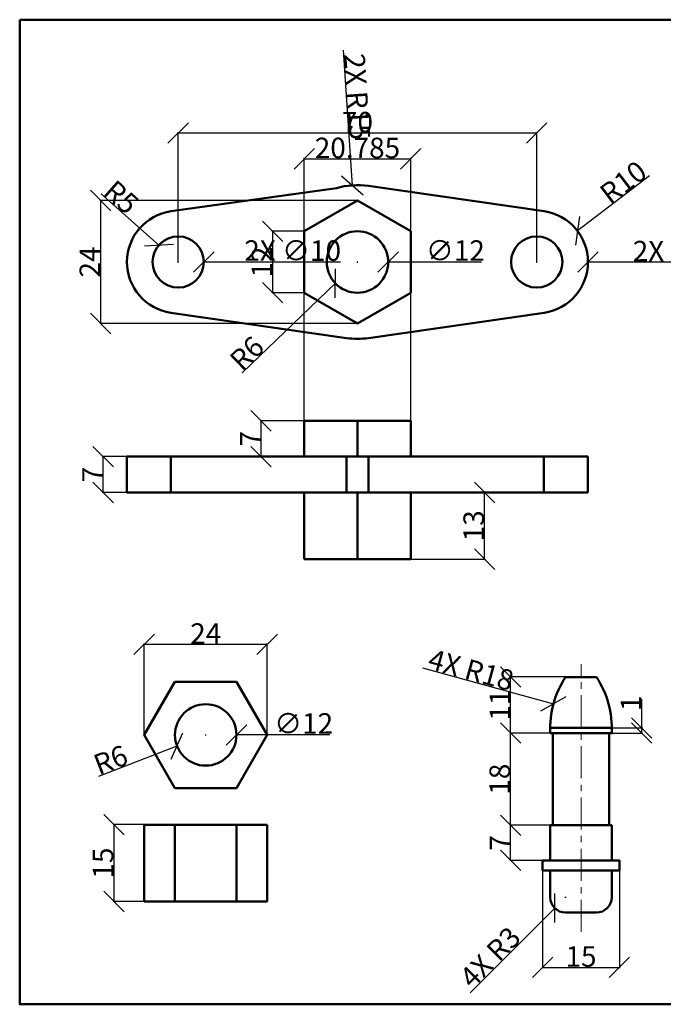
# Model space of a CAD drawing. Units: millimetres. Extents: x 4 to 224, y 3 to 195.
# Tile 1 of 2: x 4 to 129, y 3 to 195. Entities that reach past the tile are written whole.
import ezdxf

# ---------------------------------------------------------------- set-up
doc = ezdxf.new("R2010")
doc.units = ezdxf.units.MM
doc.header["$MEASUREMENT"] = 0
doc.linetypes.add('CENTER', pattern=[2, 1.25, -0.25, 0.25, -0.25])
for name, color, linetype, lineweight in [('M-CNTR', 1, 'CENTER', 18), ('M-DIMS', 2, 'Continuous', 25), ('M-OUTL', 7, 'Continuous', 50)]:
    doc.layers.add(name, color=color, linetype=linetype, lineweight=lineweight)
doc.styles.get("Standard").update_dxf_attribs({"font": 'arial.ttf'})
doc.dimstyles.get("Standard").update_dxf_attribs({"dimtxt": 4, "dimasz": 4, "dimexe": 0.18, "dimexo": 0.0625, "dimgap": 0.09, "dimtad": 1, "dimdec": 0, "dimzin": 0, "dimdsep": 46, "dimtxsty": 'Standard', "dimblk": 'OBLIQUE', "dimcen": 0.09, "dimclre": 251, "dimadec": 0, "dimazin": 0, "dimtfac": 1, "dimtdec": 0, "dimtofl": 0, "dimtmove": 0, "dimatfit": 3, "dimfxl": 1, "dimtolj": 1, "dimtzin": 0, "dimarcsym": 0})

# ---------------------------------------------------------------- blocks, each defined once
blk = doc.blocks.new('_Oblique')
at = {"color": 0, "linetype": 'ByBlock', "lineweight": -2}
blk.add_line((-0.5, -0.5), (0.5, 0.5), dxfattribs=at)
blk = doc.blocks.new('*D2')
at = {"layer": 'Defpoints', "color": 0, "transparency": 16777216}
for p in [(104.72, 173.13), (34.72, 147.94), (104.72, 147.94)]:
    blk.add_point(p, dxfattribs=at)
at = {"layer": 'M-DIMS', "color": 0, "lineweight": -2, "transparency": 16777216}
for p, q in [((34.72, 148.01), (34.72, 173.31)), ((34.72, 173.13), (104.72, 173.13)), ((104.72, 148.01), (104.72, 173.31))]:
    blk.add_line(p, q, dxfattribs=at)
at = {"layer": 'M-DIMS', "color": 0, "lineweight": -2, "transparency": 16777216, "xscale": 4, "yscale": 4, "zscale": 4, "rotation": 180}
blk.add_blockref('_Oblique', (34.72, 173.13), dxfattribs=at)
at = {"layer": 'M-DIMS', "color": 0, "lineweight": -2, "transparency": 16777216, "xscale": 4, "yscale": 4, "zscale": 4}
blk.add_blockref('_Oblique', (104.72, 173.13), dxfattribs=at)
at = {"layer": 'M-DIMS', "color": 0, "transparency": 16777216, "insert": (69.72, 175.26), "char_height": 4, "attachment_point": 5}
blk.add_mtext('\\A1;70', dxfattribs=at)
blk = doc.blocks.new('*D3')
at = {"layer": 'Defpoints', "color": 0, "transparency": 16777216}
for p in [(59.33, 153.94), (53.16, 141.94), (59.33, 141.94)]:
    blk.add_point(p, dxfattribs=at)
at = {"layer": 'M-DIMS', "color": 0, "lineweight": -2, "transparency": 16777216}
for p, q in [((59.27, 153.94), (52.98, 153.94)), ((53.16, 153.94), (53.16, 141.94)), ((59.27, 141.94), (52.98, 141.94))]:
    blk.add_line(p, q, dxfattribs=at)
at = {"layer": 'M-DIMS', "color": 0, "lineweight": -2, "transparency": 16777216, "xscale": 4, "yscale": 4, "zscale": 4}
for p, rotation in [((53.16, 153.94), 90), ((53.16, 141.94), 270)]:
    blk.add_blockref('_Oblique', p, dxfattribs=dict(at, rotation=rotation))
at = {"layer": 'M-DIMS', "color": 0, "transparency": 16777216, "insert": (51.06, 147.94), "char_height": 4, "attachment_point": 5, "rotation": 90}
blk.add_mtext('\\A1;12', dxfattribs=at)
blk = doc.blocks.new('*D4')
at = {"layer": 'Defpoints', "color": 0, "transparency": 16777216}
for p in [(69.72, 147.94), (65.4, 143.78)]:
    blk.add_point(p, dxfattribs=at)
at = {"layer": 'M-DIMS', "color": 0, "lineweight": -2, "transparency": 16777216}
for p, q in [((69.72, 147.85), (69.72, 148.03)), ((69.63, 147.94), (69.81, 147.94)), ((47.22, 126.29), (65.4, 143.78))]:
    blk.add_line(p, q, dxfattribs=at)
at = {"layer": 'M-DIMS', "color": 0, "lineweight": -2, "transparency": 16777216, "xscale": 4, "yscale": 4, "zscale": 4, "rotation": 43.89831917731966}
blk.add_blockref('_Oblique', (65.4, 143.78), dxfattribs=at)
at = {"layer": 'M-DIMS', "color": 0, "transparency": 16777216, "insert": (48.13, 130.13), "char_height": 4, "attachment_point": 5, "rotation": 43.8983}
blk.add_mtext('\\A1;R6', dxfattribs=at)
blk = doc.blocks.new('*D5')
at = {"layer": 'Defpoints', "color": 0, "transparency": 16777216}
for p in [(112.67, 154.01), (104.72, 147.94)]:
    blk.add_point(p, dxfattribs=at)
at = {"layer": 'M-DIMS', "color": 0, "lineweight": -2, "transparency": 16777216}
for p, q in [((126.76, 164.76), (112.67, 154.01)), ((104.72, 147.85), (104.72, 148.03)), ((104.63, 147.94), (104.81, 147.94))]:
    blk.add_line(p, q, dxfattribs=at)
at = {"layer": 'M-DIMS', "color": 0, "lineweight": -2, "transparency": 16777216, "xscale": 4, "yscale": 4, "zscale": 4, "rotation": 217.3494381917111}
blk.add_blockref('_Oblique', (112.67, 154.01), dxfattribs=at)
at = {"layer": 'M-DIMS', "color": 0, "transparency": 16777216, "insert": (121.6, 163.51), "char_height": 4, "attachment_point": 5, "rotation": 37.3494}
blk.add_mtext('\\A1;R10', dxfattribs=at)
blk = doc.blocks.new('*D6')
at = {"layer": 'Defpoints', "color": 0, "transparency": 16777216}
for p in [(30.97, 151.26), (34.72, 147.94)]:
    blk.add_point(p, dxfattribs=at)
at = {"layer": 'M-DIMS', "color": 0, "lineweight": -2, "transparency": 16777216}
for p, q in [((19.69, 161.23), (30.97, 151.26)), ((34.72, 147.85), (34.72, 148.03)), ((34.63, 147.94), (34.81, 147.94))]:
    blk.add_line(p, q, dxfattribs=at)
at = {"layer": 'M-DIMS', "color": 0, "lineweight": -2, "transparency": 16777216, "xscale": 4, "yscale": 4, "zscale": 4, "rotation": 318.5221166633732}
blk.add_blockref('_Oblique', (30.97, 151.26), dxfattribs=at)
at = {"layer": 'M-DIMS', "color": 0, "transparency": 16777216, "insert": (23.6, 160.61), "char_height": 4, "attachment_point": 5, "rotation": 318.5221}
blk.add_mtext('\\A1;R5', dxfattribs=at)
blk = doc.blocks.new('*D7')
at = {"layer": 'Defpoints', "color": 0, "transparency": 16777216}
for p in [(20.08, 109.94), (24.72, 109.94), (24.72, 102.94)]:
    blk.add_point(p, dxfattribs=at)
at = {"layer": 'M-DIMS', "color": 0, "lineweight": -2, "transparency": 16777216}
for p, q in [((24.66, 109.94), (19.9, 109.94)), ((20.08, 102.94), (20.08, 109.94)), ((24.66, 102.94), (19.9, 102.94))]:
    blk.add_line(p, q, dxfattribs=at)
at = {"layer": 'M-DIMS', "color": 0, "lineweight": -2, "transparency": 16777216, "xscale": 4, "yscale": 4, "zscale": 4}
for p, rotation in [((20.08, 109.94), 90), ((20.08, 102.94), 270)]:
    blk.add_blockref('_Oblique', p, dxfattribs=dict(at, rotation=rotation))
at = {"layer": 'M-DIMS', "color": 0, "transparency": 16777216, "insert": (17.99, 106.44), "char_height": 4, "attachment_point": 5, "rotation": 90}
blk.add_mtext('\\A1;7', dxfattribs=at)
blk = doc.blocks.new('*D8')
at = {"layer": 'Defpoints', "color": 0, "transparency": 16777216}
for p in [(59.33, 116.94), (50.88, 109.94), (50.88, 109.94)]:
    blk.add_point(p, dxfattribs=at)
at = {"layer": 'M-DIMS', "color": 0, "lineweight": -2, "transparency": 16777216}
for p, q in [((59.27, 116.94), (50.7, 116.94)), ((50.88, 116.94), (50.88, 109.94)), ((50.81, 109.94), (50.7, 109.94))]:
    blk.add_line(p, q, dxfattribs=at)
at = {"layer": 'M-DIMS', "color": 0, "lineweight": -2, "transparency": 16777216, "xscale": 4, "yscale": 4, "zscale": 4}
for p, rotation in [((50.88, 116.94), 90), ((50.88, 109.94), 270)]:
    blk.add_blockref('_Oblique', p, dxfattribs=dict(at, rotation=rotation))
at = {"layer": 'M-DIMS', "color": 0, "transparency": 16777216, "insert": (48.79, 113.44), "char_height": 4, "attachment_point": 5, "rotation": 90}
blk.add_mtext('\\A1;7', dxfattribs=at)
blk = doc.blocks.new('*D9')
at = {"layer": 'Defpoints', "color": 0, "transparency": 16777216}
for p in [(94.54, 102.94), (94.54, 102.94), (80.11, 89.94)]:
    blk.add_point(p, dxfattribs=at)
at = {"layer": 'M-DIMS', "color": 0, "lineweight": -2, "transparency": 16777216}
for p, q in [((94.54, 89.94), (94.54, 102.94)), ((94.6, 102.94), (94.72, 102.94)), ((80.17, 89.94), (94.72, 89.94))]:
    blk.add_line(p, q, dxfattribs=at)
at = {"layer": 'M-DIMS', "color": 0, "lineweight": -2, "transparency": 16777216, "xscale": 4, "yscale": 4, "zscale": 4}
for p, rotation in [((94.54, 102.94), 90), ((94.54, 89.94), 270)]:
    blk.add_blockref('_Oblique', p, dxfattribs=dict(at, rotation=rotation))
at = {"layer": 'M-DIMS', "color": 0, "transparency": 16777216, "insert": (92.41, 96.44), "char_height": 4, "attachment_point": 5, "rotation": 90}
blk.add_mtext('\\A1;13', dxfattribs=at)
blk = doc.blocks.new('*D22')
at = {"layer": 'Defpoints', "color": 0, "transparency": 16777216}
for p in [(52.09, 73.3), (28.09, 55.61), (52.09, 55.61)]:
    blk.add_point(p, dxfattribs=at)
at = {"layer": 'M-DIMS', "color": 0, "lineweight": -2, "transparency": 16777216}
for p, q in [((28.09, 55.67), (28.09, 73.48)), ((28.09, 73.3), (52.09, 73.3)), ((52.09, 55.67), (52.09, 73.48))]:
    blk.add_line(p, q, dxfattribs=at)
at = {"layer": 'M-DIMS', "color": 0, "lineweight": -2, "transparency": 16777216, "xscale": 4, "yscale": 4, "zscale": 4, "rotation": 180}
blk.add_blockref('_Oblique', (28.09, 73.3), dxfattribs=at)
at = {"layer": 'M-DIMS', "color": 0, "lineweight": -2, "transparency": 16777216, "xscale": 4, "yscale": 4, "zscale": 4}
blk.add_blockref('_Oblique', (52.09, 73.3), dxfattribs=at)
at = {"layer": 'M-DIMS', "color": 0, "transparency": 16777216, "insert": (40.09, 75.4), "char_height": 4, "attachment_point": 5}
blk.add_mtext('\\A1;24', dxfattribs=at)
blk = doc.blocks.new('*D23')
at = {"layer": 'Defpoints', "color": 0, "transparency": 16777216}
for p in [(40.09, 55.61), (34.5, 53.45)]:
    blk.add_point(p, dxfattribs=at)
at = {"layer": 'M-DIMS', "color": 0, "lineweight": -2, "transparency": 16777216}
for p, q in [((40, 55.61), (40.18, 55.61)), ((40.09, 55.52), (40.09, 55.7)), ((19.21, 47.57), (34.5, 53.45))]:
    blk.add_line(p, q, dxfattribs=at)
at = {"layer": 'M-DIMS', "color": 0, "lineweight": -2, "transparency": 16777216, "xscale": 4, "yscale": 4, "zscale": 4, "rotation": 21.05754839460186}
blk.add_blockref('_Oblique', (34.5, 53.45), dxfattribs=at)
at = {"layer": 'M-DIMS', "color": 0, "transparency": 16777216, "insert": (21.53, 50.75), "char_height": 4, "attachment_point": 5, "rotation": 21.0575}
blk.add_mtext('\\A1;R6', dxfattribs=at)
blk = doc.blocks.new('*D24')
at = {"layer": 'Defpoints', "color": 0, "transparency": 16777216}
for p in [(28.09, 38.09), (22.18, 23.09), (28.09, 23.09)]:
    blk.add_point(p, dxfattribs=at)
at = {"layer": 'M-DIMS', "color": 0, "lineweight": -2, "transparency": 16777216}
for p, q in [((28.03, 38.09), (22, 38.09)), ((22.18, 38.09), (22.18, 23.09)), ((28.03, 23.09), (22, 23.09))]:
    blk.add_line(p, q, dxfattribs=at)
at = {"layer": 'M-DIMS', "color": 0, "lineweight": -2, "transparency": 16777216, "xscale": 4, "yscale": 4, "zscale": 4}
for p, rotation in [((22.18, 38.09), 90), ((22.18, 23.09), 270)]:
    blk.add_blockref('_Oblique', p, dxfattribs=dict(at, rotation=rotation))
at = {"layer": 'M-DIMS', "color": 0, "transparency": 16777216, "insert": (20.05, 30.59), "char_height": 4, "attachment_point": 5, "rotation": 90}
blk.add_mtext('\\A1;15', dxfattribs=at)
blk = doc.blocks.new('*D25')
at = {"layer": 'Defpoints', "color": 0, "transparency": 16777216}
for p in [(105.86, 29.12), (120.86, 29.12), (120.86, 10.22)]:
    blk.add_point(p, dxfattribs=at)
at = {"layer": 'M-DIMS', "color": 0, "lineweight": -2, "transparency": 16777216}
for p, q in [((105.86, 29.05), (105.86, 10.04)), ((120.86, 29.05), (120.86, 10.04)), ((105.86, 10.22), (120.86, 10.22))]:
    blk.add_line(p, q, dxfattribs=at)
at = {"layer": 'M-DIMS', "color": 0, "lineweight": -2, "transparency": 16777216, "xscale": 4, "yscale": 4, "zscale": 4, "rotation": 180}
blk.add_blockref('_Oblique', (105.86, 10.22), dxfattribs=at)
at = {"layer": 'M-DIMS', "color": 0, "lineweight": -2, "transparency": 16777216, "xscale": 4, "yscale": 4, "zscale": 4}
blk.add_blockref('_Oblique', (120.86, 10.22), dxfattribs=at)
at = {"layer": 'M-DIMS', "color": 0, "transparency": 16777216, "insert": (113.36, 12.35), "char_height": 4, "attachment_point": 5}
blk.add_mtext('\\A1;15', dxfattribs=at)
blk = doc.blocks.new('*D26')
at = {"layer": 'Defpoints', "color": 0, "transparency": 16777216}
for p in [(99.62, 37.97), (107.36, 37.97), (105.86, 31.12)]:
    blk.add_point(p, dxfattribs=at)
at = {"layer": 'M-DIMS', "color": 0, "lineweight": -2, "transparency": 16777216}
for p, q in [((107.3, 37.97), (99.44, 37.97)), ((99.62, 31.12), (99.62, 37.97)), ((105.8, 31.12), (99.44, 31.12))]:
    blk.add_line(p, q, dxfattribs=at)
at = {"layer": 'M-DIMS', "color": 0, "lineweight": -2, "transparency": 16777216, "xscale": 4, "yscale": 4, "zscale": 4}
for p, rotation in [((99.62, 37.97), 90), ((99.62, 31.12), 270)]:
    blk.add_blockref('_Oblique', p, dxfattribs=dict(at, rotation=rotation))
at = {"layer": 'M-DIMS', "color": 0, "transparency": 16777216, "insert": (97.53, 34.54), "char_height": 4, "attachment_point": 5, "rotation": 90}
blk.add_mtext('\\A1;7', dxfattribs=at)
blk = doc.blocks.new('*D27')
at = {"layer": 'Defpoints', "color": 0, "transparency": 16777216}
for p in [(99.62, 55.97), (107.36, 55.97), (107.36, 37.97)]:
    blk.add_point(p, dxfattribs=at)
at = {"layer": 'M-DIMS', "color": 0, "lineweight": -2, "transparency": 16777216}
for p, q in [((107.3, 55.97), (99.44, 55.97)), ((99.62, 37.97), (99.62, 55.97)), ((107.3, 37.97), (99.44, 37.97))]:
    blk.add_line(p, q, dxfattribs=at)
at = {"layer": 'M-DIMS', "color": 0, "lineweight": -2, "transparency": 16777216, "xscale": 4, "yscale": 4, "zscale": 4}
for p, rotation in [((99.62, 55.97), 90), ((99.62, 37.97), 270)]:
    blk.add_blockref('_Oblique', p, dxfattribs=dict(at, rotation=rotation))
at = {"layer": 'M-DIMS', "color": 0, "transparency": 16777216, "insert": (97.49, 46.97), "char_height": 4, "attachment_point": 5, "rotation": 90}
blk.add_mtext('\\A1;18', dxfattribs=at)
blk = doc.blocks.new('*D28')
at = {"layer": 'Defpoints', "color": 0, "transparency": 16777216}
for p in [(99.62, 66.92), (110.36, 66.92), (107.36, 55.97)]:
    blk.add_point(p, dxfattribs=at)
at = {"layer": 'M-DIMS', "color": 0, "lineweight": -2, "transparency": 16777216}
for p, q in [((110.3, 66.92), (99.44, 66.92)), ((99.62, 55.97), (99.62, 66.92)), ((107.3, 55.97), (99.44, 55.97))]:
    blk.add_line(p, q, dxfattribs=at)
at = {"layer": 'M-DIMS', "color": 0, "lineweight": -2, "transparency": 16777216, "xscale": 4, "yscale": 4, "zscale": 4}
for p, rotation in [((99.62, 66.92), 90), ((99.62, 55.97), 270)]:
    blk.add_blockref('_Oblique', p, dxfattribs=dict(at, rotation=rotation))
at = {"layer": 'M-DIMS', "color": 0, "transparency": 16777216, "insert": (97.52, 61.44), "char_height": 4, "attachment_point": 5, "rotation": 90}
blk.add_mtext('\\A1;11', dxfattribs=at)
blk = doc.blocks.new('*D29')
at = {"layer": 'Defpoints', "color": 0, "transparency": 16777216}
for p in [(119.36, 56.97), (119.36, 55.97), (125.22, 56.97)]:
    blk.add_point(p, dxfattribs=at)
at = {"layer": 'M-DIMS', "color": 0, "lineweight": -2, "transparency": 16777216}
for p, q in [((125.22, 56.97), (125.22, 62.62)), ((119.42, 56.97), (125.4, 56.97)), ((119.42, 55.97), (125.4, 55.97)), ((125.22, 55.97), (125.22, 56.97))]:
    blk.add_line(p, q, dxfattribs=at)
at = {"layer": 'M-DIMS', "color": 0, "lineweight": -2, "transparency": 16777216, "xscale": 4, "yscale": 4, "zscale": 4}
for p, rotation in [((125.22, 56.97), 90), ((125.22, 55.97), 270)]:
    blk.add_blockref('_Oblique', p, dxfattribs=dict(at, rotation=rotation))
at = {"layer": 'M-DIMS', "color": 0, "transparency": 16777216, "insert": (123.13, 61.79), "char_height": 4, "attachment_point": 5, "rotation": 90}
blk.add_mtext('\\A1;1', dxfattribs=at)
blk = doc.blocks.new('*D37')
at = {"layer": 'Defpoints', "color": 0, "transparency": 16777216}
for p in [(69.72, 159.94), (19.57, 135.94), (69.72, 135.94)]:
    blk.add_point(p, dxfattribs=at)
at = {"layer": 'M-DIMS', "color": 251, "lineweight": -2, "transparency": 16777216}
for p, q in [((69.66, 159.94), (19.39, 159.94)), ((69.66, 135.94), (19.39, 135.94))]:
    blk.add_line(p, q, dxfattribs=at)
at = {"layer": 'M-DIMS', "color": 0, "lineweight": -2, "transparency": 16777216}
blk.add_line((19.57, 159.94), (19.57, 135.94), dxfattribs=at)
at = {"layer": 'M-DIMS', "color": 0, "lineweight": -2, "transparency": 16777216, "xscale": 4, "yscale": 4, "zscale": 4}
for p, rotation in [((19.57, 159.94), 90), ((19.57, 135.94), 270)]:
    blk.add_blockref('_Oblique', p, dxfattribs=dict(at, rotation=rotation))
at = {"layer": 'M-DIMS', "color": 0, "transparency": 16777216, "insert": (17.47, 147.94), "char_height": 4, "attachment_point": 5, "rotation": 90}
blk.add_mtext('\\A1;24', dxfattribs=at)
blk = doc.blocks.new('*D38')
at = {"layer": 'Defpoints', "color": 0, "transparency": 16777216}
for p in [(80.11, 168.08), (59.33, 116.94), (80.11, 116.94)]:
    blk.add_point(p, dxfattribs=at)
at = {"layer": 'M-DIMS', "color": 251, "lineweight": -2, "transparency": 16777216}
for p, q in [((59.33, 117), (59.33, 168.26)), ((80.11, 117), (80.11, 168.26))]:
    blk.add_line(p, q, dxfattribs=at)
at = {"layer": 'M-DIMS', "color": 0, "lineweight": -2, "transparency": 16777216}
blk.add_line((59.33, 168.08), (80.11, 168.08), dxfattribs=at)
at = {"layer": 'M-DIMS', "color": 0, "lineweight": -2, "transparency": 16777216, "xscale": 4, "yscale": 4, "zscale": 4, "rotation": 180}
blk.add_blockref('_Oblique', (59.33, 168.08), dxfattribs=at)
at = {"layer": 'M-DIMS', "color": 0, "lineweight": -2, "transparency": 16777216, "xscale": 4, "yscale": 4, "zscale": 4}
blk.add_blockref('_Oblique', (80.11, 168.08), dxfattribs=at)
at = {"layer": 'M-DIMS', "color": 0, "transparency": 16777216, "insert": (69.72, 170.22), "char_height": 4, "attachment_point": 5}
blk.add_mtext('\\A1;20.785', dxfattribs=at)
blk = doc.blocks.new('*D40')
at = {"layer": 'Defpoints', "color": 0, "transparency": 16777216}
for p in [(29.72, 147.95), (39.72, 147.94)]:
    blk.add_point(p, dxfattribs=at)
at = {"layer": 'M-DIMS', "color": 251, "lineweight": -2, "transparency": 16777216}
for p, q in [((34.72, 147.85), (34.72, 148.03)), ((34.63, 147.94), (34.81, 147.94))]:
    blk.add_line(p, q, dxfattribs=at)
at = {"layer": 'M-DIMS', "color": 0, "lineweight": -2, "transparency": 16777216}
blk.add_line((66.42, 147.92), (39.72, 147.94), dxfattribs=at)
at = {"layer": 'M-DIMS', "color": 0, "lineweight": -2, "transparency": 16777216, "xscale": 4, "yscale": 4, "zscale": 4, "rotation": 179.9524330357494}
blk.add_blockref('_Oblique', (39.72, 147.94), dxfattribs=at)
at = {"layer": 'M-DIMS', "color": 0, "transparency": 16777216, "insert": (57.07, 150.17), "char_height": 4, "attachment_point": 5, "rotation": 359.9524}
blk.add_mtext('\\A1;2X ∅10', dxfattribs=at)
blk = doc.blocks.new('*D41')
at = {"layer": 'Defpoints', "color": 0, "transparency": 16777216}
for p in [(63.72, 147.95), (75.72, 147.94)]:
    blk.add_point(p, dxfattribs=at)
at = {"layer": 'M-DIMS', "color": 251, "lineweight": -2, "transparency": 16777216}
for p, q in [((69.72, 147.85), (69.72, 148.03)), ((69.63, 147.94), (69.81, 147.94))]:
    blk.add_line(p, q, dxfattribs=at)
at = {"layer": 'M-DIMS', "color": 0, "lineweight": -2, "transparency": 16777216}
blk.add_line((93.94, 147.93), (75.72, 147.94), dxfattribs=at)
at = {"layer": 'M-DIMS', "color": 0, "lineweight": -2, "transparency": 16777216, "xscale": 4, "yscale": 4, "zscale": 4, "rotation": 179.9603608629846}
blk.add_blockref('_Oblique', (75.72, 147.94), dxfattribs=at)
at = {"layer": 'M-DIMS', "color": 0, "transparency": 16777216, "insert": (88.83, 150.18), "char_height": 4, "attachment_point": 5, "rotation": 359.9604}
blk.add_mtext('\\A1;∅12', dxfattribs=at)
blk = doc.blocks.new('*D42')
at = {"layer": 'Defpoints', "color": 0, "transparency": 16777216}
for p in [(104.72, 147.94), (114.72, 147.94)]:
    blk.add_point(p, dxfattribs=at)
at = {"layer": 'M-DIMS', "color": 251, "lineweight": -2, "transparency": 16777216}
for p, q in [((104.72, 147.85), (104.72, 148.03)), ((104.63, 147.94), (104.81, 147.94))]:
    blk.add_line(p, q, dxfattribs=at)
at = {"layer": 'M-DIMS', "color": 0, "lineweight": -2, "transparency": 16777216}
blk.add_line((141.11, 147.93), (114.72, 147.94), dxfattribs=at)
at = {"layer": 'M-DIMS', "color": 0, "lineweight": -2, "transparency": 16777216, "xscale": 4, "yscale": 4, "zscale": 4, "rotation": 179.9762165209119}
blk.add_blockref('_Oblique', (114.72, 147.94), dxfattribs=at)
at = {"layer": 'M-DIMS', "color": 0, "transparency": 16777216, "insert": (131.91, 150.07), "char_height": 4, "attachment_point": 5, "rotation": 359.9762}
blk.add_mtext('\\A1;2X R10', dxfattribs=at)
blk = doc.blocks.new('*D43')
at = {"layer": 'Defpoints', "color": 0, "transparency": 16777216}
for p in [(68.71, 162.91), (69.72, 147.94)]:
    blk.add_point(p, dxfattribs=at)
at = {"layer": 'M-DIMS', "color": 0, "lineweight": -2, "transparency": 16777216}
blk.add_line((66.93, 189.28), (68.71, 162.91), dxfattribs=at)
at = {"layer": 'M-DIMS', "color": 251, "lineweight": -2, "transparency": 16777216}
for p, q in [((69.72, 147.85), (69.72, 148.03)), ((69.63, 147.94), (69.81, 147.94))]:
    blk.add_line(p, q, dxfattribs=at)
at = {"layer": 'M-DIMS', "color": 0, "lineweight": -2, "transparency": 16777216, "xscale": 4, "yscale": 4, "zscale": 4, "rotation": 273.8605650789521}
blk.add_blockref('_Oblique', (68.71, 162.91), dxfattribs=at)
at = {"layer": 'M-DIMS', "color": 0, "transparency": 16777216, "insert": (69.68, 180.23), "char_height": 4, "attachment_point": 5, "rotation": 273.8606}
blk.add_mtext('\\A1;2X R15', dxfattribs=at)
blk = doc.blocks.new('*D45')
at = {"layer": 'Defpoints', "color": 0, "transparency": 16777216}
for p in [(34.09, 55.61), (46.09, 55.61)]:
    blk.add_point(p, dxfattribs=at)
at = {"layer": 'M-DIMS', "color": 251, "lineweight": -2, "transparency": 16777216}
for p, q in [((40, 55.61), (40.18, 55.61)), ((40.09, 55.52), (40.09, 55.7))]:
    blk.add_line(p, q, dxfattribs=at)
at = {"layer": 'M-DIMS', "color": 0, "lineweight": -2, "transparency": 16777216}
blk.add_line((64.32, 55.61), (46.09, 55.61), dxfattribs=at)
at = {"layer": 'M-DIMS', "color": 0, "lineweight": -2, "transparency": 16777216, "xscale": 4, "yscale": 4, "zscale": 4, "rotation": 179.9944136615151}
blk.add_blockref('_Oblique', (46.09, 55.61), dxfattribs=at)
at = {"layer": 'M-DIMS', "color": 0, "transparency": 16777216, "insert": (59.21, 57.85), "char_height": 4, "attachment_point": 5, "rotation": 359.9944}
blk.add_mtext('\\A1;∅12', dxfattribs=at)
blk = doc.blocks.new('*D46')
at = {"layer": 'Defpoints', "color": 0, "transparency": 16777216}
for p in [(107.98, 61.69), (125.33, 56.93)]:
    blk.add_point(p, dxfattribs=at)
at = {"layer": 'M-DIMS', "color": 0, "lineweight": -2, "transparency": 16777216}
blk.add_line((82.42, 68.7), (107.98, 61.69), dxfattribs=at)
at = {"layer": 'M-DIMS', "color": 251, "lineweight": -2, "transparency": 16777216}
for p, q in [((125.24, 56.93), (125.42, 56.93)), ((125.33, 56.84), (125.33, 57.02))]:
    blk.add_line(p, q, dxfattribs=at)
at = {"layer": 'M-DIMS', "color": 0, "lineweight": -2, "transparency": 16777216, "xscale": 4, "yscale": 4, "zscale": 4, "rotation": 344.6657255947465}
blk.add_blockref('_Oblique', (107.98, 61.69), dxfattribs=at)
at = {"layer": 'M-DIMS', "color": 0, "transparency": 16777216, "insert": (91.9, 68.31), "char_height": 4, "attachment_point": 5, "rotation": 344.6657}
blk.add_mtext('\\A1;4X R18', dxfattribs=at)
blk = doc.blocks.new('*D47')
at = {"layer": 'Defpoints', "color": 0, "transparency": 16777216}
for p in [(110.36, 23.92), (108.24, 21.8)]:
    blk.add_point(p, dxfattribs=at)
at = {"layer": 'M-DIMS', "color": 251, "lineweight": -2, "transparency": 16777216}
for p, q in [((110.27, 23.92), (110.45, 23.92)), ((110.36, 23.83), (110.36, 24.01))]:
    blk.add_line(p, q, dxfattribs=at)
at = {"layer": 'M-DIMS', "color": 0, "lineweight": -2, "transparency": 16777216}
blk.add_line((91.69, 5.27), (108.24, 21.8), dxfattribs=at)
at = {"layer": 'M-DIMS', "color": 0, "lineweight": -2, "transparency": 16777216, "xscale": 4, "yscale": 4, "zscale": 4, "rotation": 44.95188258666079}
blk.add_blockref('_Oblique', (108.24, 21.8), dxfattribs=at)
at = {"layer": 'M-DIMS', "color": 0, "transparency": 16777216, "insert": (95.62, 12.22), "char_height": 4, "attachment_point": 5, "rotation": 44.9519}
blk.add_mtext('\\A1;4X R3', dxfattribs=at)

msp = doc.modelspace()

# ---------------------------------------------------------------- linework, layer by layer
at = {"layer": 'M-CNTR', "ltscale": 5}
msp.add_line((113.3604, 17.1404), (113.3604, 69.4089), dxfattribs=at)
at = {"layer": 'M-OUTL'}
for p, q in [((33.3328, 157.8475), (65.5987, 162.3669)), ((71.8628, 162.7903), (106.1485, 157.8416)), ((33.2913, 138.0467), (67.5771, 133.098)), ((71.8628, 133.098), (106.1485, 138.0467)), ((59.3276, 116.9392), (59.3276, 109.9392)), ((59.3276, 116.9392), (80.1122, 116.9392)), ((69.7199, 116.9392), (69.7199, 109.9392)), ((80.1122, 116.9392), (80.1122, 109.9392)), ((24.7199, 102.9392), (24.7199, 109.9392)), ((24.7199, 109.9392), (114.7199, 109.9392)), ((33.3115, 102.9392), (33.3115, 109.9392)), ((67.5558, 102.9392), (67.5558, 109.9392)), ((71.8415, 102.9392), (71.8415, 109.9392)), ((106.1272, 102.9392), (106.1272, 109.9392)), ((114.7199, 102.9392), (114.7199, 109.9392)), ((24.7199, 102.9392), (114.7199, 102.9392)), ((59.3276, 102.9392), (59.3276, 89.9392)), ((69.7199, 102.9392), (69.7199, 89.9392)), ((80.1122, 102.9392), (80.1122, 89.9392)), ((59.3276, 89.9392), (80.1122, 89.9392)), ((110.3604, 66.9169), (116.3604, 66.9169)), ((107.3604, 56.9669), (119.3604, 56.9669)), ((107.3604, 55.9669), (119.3604, 55.9669)), ((107.8604, 37.9669), (107.8604, 55.9669)), ((118.8604, 37.9669), (118.8604, 55.9669)), ((28.0945, 38.0878), (28.0945, 23.0878)), ((28.0945, 38.0878), (52.0945, 38.0878)), ((34.0945, 38.0878), (34.0945, 23.0878)), ((46.0945, 38.0878), (46.0945, 23.0878)), ((52.0945, 38.0878), (52.0945, 23.0878)), ((107.3604, 31.1169), (107.3604, 37.9669)), ((107.3604, 37.9669), (119.3604, 37.9669)), ((119.3604, 31.1169), (119.3604, 37.9669)), ((107.3604, 23.9169), (107.3604, 29.1169)), ((119.3604, 23.9169), (119.3604, 29.1169)), ((28.0945, 23.0878), (52.0945, 23.0878)), ((110.3604, 20.9169), (116.3604, 20.9169))]:
    msp.add_line(p, q, dxfattribs=at)
for points in [[(3.7754, 195.2521), (224.2583, 195.2521), (224.2583, 3.0162), (3.7754, 3.0162)], [(59.3276, 141.9442), (69.7199, 135.9442), (80.1122, 141.9442), (80.1122, 153.9442), (69.7199, 159.9442), (59.3276, 153.9442)], [(34.0945, 66.0029), (28.0945, 55.6106), (34.0945, 45.2183), (46.0945, 45.2183), (52.0945, 55.6106), (46.0945, 66.0029)], [(105.8604, 31.1169), (120.8604, 31.1169), (120.8604, 29.1169), (105.8604, 29.1169)]]:
    msp.add_lwpolyline(points, close=True, dxfattribs=at)
for centre, radius in [((69.7199, 147.9442), 6), ((34.7199, 147.9442), 5), ((104.7199, 147.9442), 5), ((40.0945, 55.6106), 6)]:
    msp.add_circle(centre, radius, dxfattribs=at)
for centre, radius, start, end in [((69.7199, 147.9442), 15, 81.786789, 105.946867), ((34.7199, 147.9442), 10, 97.973434, 261.786789), ((104.7199, 147.9442), 10, 278.213211, 81.786789), ((69.7199, 147.9442), 15, 261.786789, 278.213211), ((125.3347, 56.9284), 18, 146.294997, 183.061983), ((101.3861, 56.9284), 18, 356.938017, 33.705003), ((110.3604, 23.9169), 3, 180, 270), ((116.3604, 23.9169), 3, 270, 0)]:
    msp.add_arc(centre, radius, start, end, dxfattribs=at)

# ---------------------------------------------------------------- dimensions: what is measured, and where the dimension line sits
at = {"layer": 'M-DIMS'}
for center, mpoint, text, picture, middle in [((69.7199, 147.9442), (68.71, 162.9101), '2X <>', '*D43', (69.6783, 180.2301)), ((104.7199, 147.9442), (114.7199, 147.94), '2X <>', '*D42', (131.9145, 150.0652)), ((125.3347, 56.9284), (107.9756, 61.6885), '4X <>', '*D46', (91.9026, 68.3069)), ((110.3604, 23.9169), (108.2373, 21.7973), '4X <>', '*D47', (95.6239, 12.22))]:
    dim = msp.add_radius_dim(center=center, mpoint=mpoint, text=text, dimstyle='Standard', override={"dimdec": 0, "dimlfac": 1, "dimrnd": 0, "dimzin": 0, "dimdsep": 46, "dimlunit": 2}, dxfattribs=at)
    dim.commit()
    dim.dimension.update_dxf_attribs({"geometry": picture, "text_midpoint": middle})
for base, p1, p2, override, picture, middle in [((104.7199, 173.1324), (34.7199, 147.9442), (104.7199, 147.9442), {"dimclrd": 0, "dimclre": 0, "dimclrt": 0}, '*D2', (69.7199, 175.2647)), ((80.1122, 168.0834), (59.3276, 116.9392), (80.1122, 116.9392), {"dimdec": 3, "dimlfac": 1, "dimrnd": 0, "dimzin": 0, "dimdsep": 46, "dimlunit": 2}, '*D38', (69.7199, 170.2157)), ((52.0945, 73.301), (28.0945, 55.6106), (52.0945, 55.6106), {"dimclrd": 0, "dimclre": 0, "dimclrt": 0}, '*D22', (40.0945, 75.3992)), ((120.8604, 10.2166), (105.8604, 29.1169), (120.8604, 29.1169), {"dimclrd": 0, "dimclre": 0, "dimclrt": 0}, '*D25', (113.3604, 12.3489))]:
    dim = msp.add_linear_dim(base=base, p1=p1, p2=p2, dimstyle='Standard', override=override, dxfattribs=at)
    dim.commit()
    dim.dimension.update_dxf_attribs({"geometry": picture, "text_midpoint": middle})
dim = msp.add_radius_dim(center=(104.7199, 147.9442), mpoint=(112.6694, 154.0109), dimstyle='Standard', override={"dimclrd": 0, "dimclre": 0, "dimclrt": 0}, dxfattribs=at)
dim.commit()
dim.dimension.update_dxf_attribs({"geometry": '*D5', "text_midpoint": (121.6006, 163.5091)})
for center, mpoint, picture, middle in [((34.7199, 147.9442), (30.9739, 151.2558), '*D6', (22.1882, 159.0227)), ((69.7199, 147.9442), (65.3965, 143.7839), '*D4', (49.6091, 128.5922)), ((40.0945, 55.6106), (34.4952, 53.4548), '*D23', (22.3002, 48.7595))]:
    dim = msp.add_radius_dim(center=center, mpoint=mpoint, dimstyle='Standard', override={"dimclrd": 0, "dimclre": 0, "dimclrt": 0}, dxfattribs=at)
    dim.commit()
    dim.dimension.update_dxf_attribs({"geometry": picture, "text_midpoint": middle, "dimtype": 164})
for base, p1, p2, override, picture, middle in [((19.5699, 135.9442), (69.7199, 159.9442), (69.7199, 135.9442), {"dimdec": 0, "dimlfac": 1, "dimrnd": 0, "dimzin": 0, "dimdsep": 46, "dimlunit": 2}, '*D37', (17.4718, 147.9442)), ((53.163, 141.9442), (59.3276, 153.9442), (59.3276, 141.9442), {"dimclrd": 0, "dimclre": 0, "dimclrt": 0}, '*D3', (51.0648, 147.9442)), ((50.8755, 109.9392), (59.3276, 116.9392), (50.8755, 109.9392), {"dimclrd": 0, "dimclre": 0, "dimclrt": 0}, '*D8', (48.7855, 113.4392)), ((20.0839, 109.9392), (24.7199, 102.9392), (24.7199, 109.9392), {"dimclrd": 0, "dimclre": 0, "dimclrt": 0}, '*D7', (17.9939, 106.4392)), ((94.5405, 102.9392), (80.1122, 89.9392), (94.5405, 102.9392), {"dimclrd": 0, "dimclre": 0, "dimclrt": 0}, '*D9', (92.4069, 96.4392)), ((99.6181, 66.9169), (107.3604, 55.9669), (110.3604, 66.9169), {"dimclrd": 0, "dimclre": 0, "dimclrt": 0}, '*D28', (97.5199, 61.4419)), ((125.2245, 56.9669), (119.3604, 55.9669), (119.3604, 56.9669), {"dimclrd": 0, "dimclre": 0, "dimclrt": 0}, '*D29', (123.1263, 61.7936)), ((99.6181, 55.9669), (107.3604, 37.9669), (107.3604, 55.9669), {"dimclrd": 0, "dimclre": 0, "dimclrt": 0}, '*D27', (97.4858, 46.9669)), ((22.1775, 23.0878), (28.0945, 38.0878), (28.0945, 23.0878), {"dimclrd": 0, "dimclre": 0, "dimclrt": 0}, '*D24', (20.0452, 30.5878)), ((99.6181, 37.9669), (105.8604, 31.1169), (107.3604, 37.9669), {"dimclrd": 0, "dimclre": 0, "dimclrt": 0}, '*D26', (97.5281, 34.5419))]:
    dim = msp.add_linear_dim(base=base, p1=p1, p2=p2, angle=90, dimstyle='Standard', override=override, dxfattribs=at)
    dim.commit()
    dim.dimension.update_dxf_attribs({"geometry": picture, "text_midpoint": middle})
dim = msp.add_diameter_dim_2p(p1=(29.7199, 147.9483), p2=(39.7199, 147.94), text='2X <>', dimstyle='Standard', override={"dimdec": 0, "dimlfac": 1, "dimrnd": 0, "dimzin": 0, "dimdsep": 46, "dimlunit": 2}, dxfattribs=at)
dim.commit()
dim.dimension.update_dxf_attribs({"geometry": '*D40', "text_midpoint": (57.0691, 147.9256), "dimtype": 163})
for p1, p2, picture, middle in [((63.7199, 147.9483), (75.7199, 147.94), '*D41', (88.8304, 147.9309)), ((34.0945, 55.6112), (46.0945, 55.61), '*D45', (59.205, 55.6087))]:
    dim = msp.add_diameter_dim_2p(p1=p1, p2=p2, dimstyle='Standard', override={"dimdec": 0, "dimlfac": 1, "dimrnd": 0, "dimzin": 0, "dimdsep": 46, "dimlunit": 2}, dxfattribs=at)
    dim.commit()
    dim.dimension.update_dxf_attribs({"geometry": picture, "text_midpoint": middle, "dimtype": 163})

doc.saveas('drawing.dxf')
